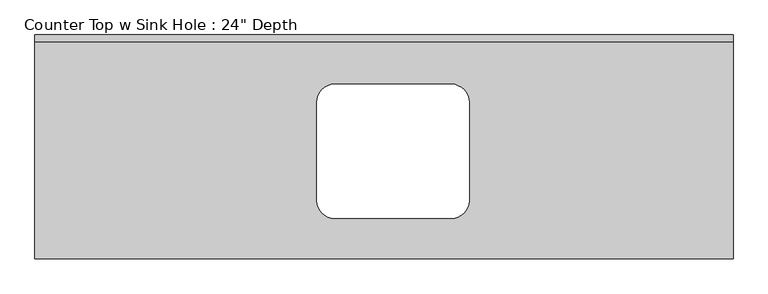
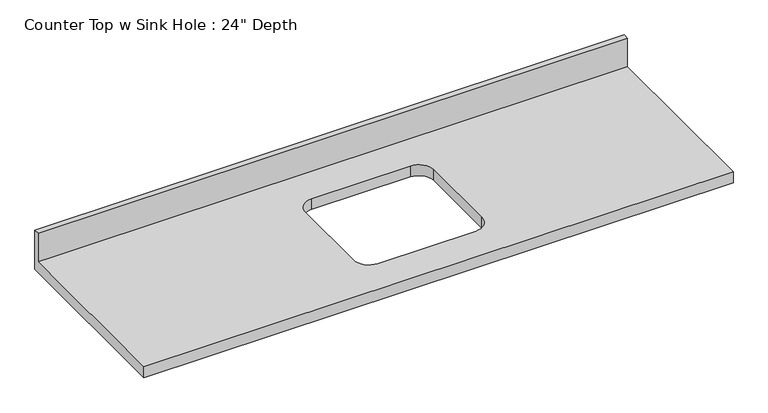
"""IFC4 building model written with IfcOpenShell, lengths in millimetres: furniture geometry."""

from ifc_helpers import new_model, si_unit, frame, origin, place, context, project, spatial, polyline, circle_curve, source, transform, mapped, element, save
from ifc_brep_helpers import plane_surface, revolved_surface, advanced_brep


def furniture_c6510c7c(model_context):
    return source(origin(), model_context, "Body", "AdvancedBrep", [
        advanced_brep(
        [(-1200.4622951, -635.0, 914.4), (780.7377049, -635.0, 914.4), (780.7377049, -19.05, 914.4), (-1200.4622951, -19.05, 914.4), (-349.5622951, -139.7, 914.4), (-19.3622951, -139.7, 914.4), (31.4377049, -190.5, 914.4), (31.4377049, -469.9, 914.4), (-19.3622951, -520.7, 914.4), (-349.5622951, -520.7, 914.4), (-400.3622951, -469.9, 914.4), (-400.3622951, -190.5, 914.4), (780.7377049, 0.0, 876.3), (780.7377049, -635.0, 876.3), (-1200.4622951, -635.0, 876.3), (-1200.4622951, 0.0, 876.3), (-19.3622951, -139.7, 876.3), (-349.5622951, -139.7, 876.3), (-400.3622951, -190.5, 876.3), (-400.3622951, -469.9, 876.3), (-349.5622951, -520.7, 876.3), (-19.3622951, -520.7, 876.3), (31.4377049, -469.9, 876.3), (31.4377049, -190.5, 876.3), (-1200.4622951, 0.0, 1016.0), (780.7377049, 0.0, 1016.0), (-1200.4622951, -19.05, 1016.0), (780.7377049, -19.05, 1016.0)],
        [
            (0, 1),
            (1, 2),
            (2, 3),
            (3, 0),
            (4, 5),
            (5, 6, circle_curve(frame((-19.3622951, -190.5, 914.4), z_axis=(0.0, 0.0, -1.0), x_axis=(1.0, 0.0, 0.0)), 50.8)),
            (6, 7),
            (7, 8, circle_curve(frame((-19.3622951, -469.9, 914.4), z_axis=(0.0, 0.0, -1.0), x_axis=(1.0, 0.0, 0.0)), 50.8)),
            (8, 9),
            (9, 10, circle_curve(frame((-349.5622951, -469.9, 914.4), z_axis=(0.0, 0.0, -1.0), x_axis=(1.0, 0.0, 0.0)), 50.8)),
            (10, 11),
            (11, 4, circle_curve(frame((-349.5622951, -190.5, 914.4), z_axis=(0.0, 0.0, -1.0), x_axis=(1.0, 0.0, 0.0)), 50.8)),
            (12, 13),
            (13, 14),
            (14, 15),
            (15, 12),
            (16, 17),
            (17, 18, circle_curve(frame((-349.5622951, -190.5, 876.3), z_axis=(0.0, 0.0, 1.0), x_axis=(1.0, 0.0, 0.0)), 50.8)),
            (18, 19),
            (19, 20, circle_curve(frame((-349.5622951, -469.9, 876.3), z_axis=(0.0, 0.0, 1.0), x_axis=(1.0, 0.0, 0.0)), 50.8)),
            (20, 21),
            (21, 22, circle_curve(frame((-19.3622951, -469.9, 876.3), z_axis=(0.0, 0.0, 1.0), x_axis=(1.0, 0.0, 0.0)), 50.8)),
            (22, 23),
            (23, 16, circle_curve(frame((-19.3622951, -190.5, 876.3), z_axis=(0.0, 0.0, 1.0), x_axis=(1.0, 0.0, 0.0)), 50.8)),
            (15, 24),
            (24, 25),
            (25, 12),
            (14, 0),
            (3, 26),
            (26, 24),
            (13, 1),
            (25, 27),
            (27, 2),
            (4, 17),
            (16, 5),
            (11, 18),
            (10, 19),
            (9, 20),
            (8, 21),
            (7, 22),
            (6, 23),
            (26, 27),
        ],
        [
            plane_surface(frame((-1200.4622951, 0.0, 914.4), z_axis=(0.0, 0.0, 1.0), x_axis=(-1.0, 0.0, 0.0))),
            plane_surface(frame((-1200.4622951, 0.0, 876.3), z_axis=(0.0, 0.0, -1.0), x_axis=(1.0, 0.0, 0.0))),
            plane_surface(frame((780.7377049, 0.0, 914.4), z_axis=(0.0, 1.0, 0.0), x_axis=(0.0, 0.0, -1.0))),
            plane_surface(frame((-1200.4622951, 0.0, 914.4), z_axis=(-1.0, 0.0, 0.0), x_axis=(0.0, 0.0, -1.0))),
            plane_surface(frame((-1200.4622951, -635.0, 914.4), z_axis=(0.0, -1.0, 0.0), x_axis=(0.0, 0.0, -1.0))),
            plane_surface(frame((780.7377049, -635.0, 914.4), z_axis=(1.0, 0.0, 0.0), x_axis=(0.0, 0.0, -1.0))),
            plane_surface(frame((-19.3622951, -139.7, 914.4), z_axis=(0.0, -1.0, 0.0), x_axis=(0.0, 0.0, -1.0))),
            revolved_surface(polyline([(-298.76229509999996, -190.5, 914.4), (-298.76229509999996, -190.5, 876.3)]), (-349.5622951, -190.5, 876.3), (0.0, 0.0, 1.0)),
            plane_surface(frame((-400.3622951, -190.5, 914.4), z_axis=(1.0, 0.0, 0.0), x_axis=(0.0, 0.0, -1.0))),
            revolved_surface(polyline([(-298.76229509999996, -469.9, 914.4), (-298.76229509999996, -469.9, 876.3)]), (-349.5622951, -469.9, 876.3), (0.0, 0.0, 1.0)),
            plane_surface(frame((-349.5622951, -520.7, 914.4), z_axis=(0.0, 1.0, 0.0), x_axis=(0.0, 0.0, -1.0))),
            revolved_surface(polyline([(31.437704899999996, -469.9, 914.4), (31.437704899999996, -469.9, 876.3)]), (-19.3622951, -469.9, 876.3), (0.0, 0.0, 1.0)),
            plane_surface(frame((31.4377049, -469.9, 914.4), z_axis=(-1.0, 0.0, 0.0), x_axis=(0.0, 0.0, -1.0))),
            revolved_surface(polyline([(31.437704899999996, -190.5, 914.4), (31.437704899999996, -190.5, 876.3)]), (-19.3622951, -190.5, 876.3), (0.0, 0.0, 1.0)),
            plane_surface(frame((-1200.4622951, 0.0, 1016.0), z_axis=(0.0, 0.0, 1.0), x_axis=(0.0, -1.0, 0.0))),
            plane_surface(frame((-1200.4622951, -19.05, 1016.0), z_axis=(0.0, -1.0, 0.0), x_axis=(0.0, 0.0, -1.0))),
        ],
        [
            (0, [[1, 2, 3, 4], [5, 6, 7, 8, 9, 10, 11, 12]]),
            (1, [[13, 14, 15, 16], [17, 18, 19, 20, 21, 22, 23, 24]]),
            (2, [[-16, 25, 26, 27]]),
            (3, [[-15, 28, -4, 29, 30, -25]]),
            (4, [[-1, -28, -14, 31]]),
            (5, [[-13, -27, 32, 33, -2, -31]]),
            (6, [[34, -17, 35, -5]]),
            (7, [[-34, -12, 36, -18]]),
            (8, [[-36, -11, 37, -19]]),
            (9, [[-37, -10, 38, -20]]),
            (10, [[-38, -9, 39, -21]]),
            (11, [[-39, -8, 40, -22]]),
            (12, [[-40, -7, 41, -23]]),
            (13, [[-35, -24, -41, -6]]),
            (14, [[-30, 42, -32, -26]]),
            (15, [[-42, -29, -3, -33]]),
        ],
    ),
    ])


if __name__ == "__main__":
    model = new_model("IFC4")
    model_context = context("Model", 3, world=origin())
    ifc_project = project(units=[si_unit("LENGTHUNIT", "METRE", prefix="MILLI")], contexts=[model_context])
    site = spatial("IfcSite", under=ifc_project)
    building = spatial("IfcBuilding", under=site)
    placement = place(None, origin())
    furniture_shape = furniture_c6510c7c(model_context)
    element("IfcFurniture", 1, ObjectType="Counter Top w Sink Hole : 24\" Depth", at=placement, inside=building, context=model_context, shape_type="MappedRepresentation", body=[
        mapped(furniture_shape, transform((0.0, 0.0, 0.0), x_axis=(1.0, 0.0, 0.0), y_axis=(0.0, 1.0, 0.0), z_axis=(0.0, 0.0, 1.0))),
    ])
    save(model, "model.ifc")

# Revit data of these elements
# Type "Counter Top w Sink Hole : 24\" Depth"
#   Assembly Code = "C1030400"
#   Counter Thickness = 0' - 1 1/2"
#   Depth = 2' - 1"
#   Height = 3' - 0"
#   Length [instance default] = 8' - 0"
#   Sink Location [instance default] = 2' - 0"
#   Sink Location To Wall [instance default] = 0' - 6"
#   Sink Opening Depth [instance default] = 1' - 3"
#   Sink Opening Width [instance default] = 2' - 3"
#   Counter Top Material = none
#   Default Elevation = 0
# Element 1 (IfcFurniture, "Counter Top w Sink Hole : 24\" Depth")
#   Length = 6' - 6"
#   Sink Location = 3' - 4"
#   Sink Opening Depth = 1' - 2"
#   Sink Opening Width = 1' - 4"
#   Materials on its faces: "Counter Top"
# Materials
#   "Counter Top": class "Wood", colour RGB 226 177 128, transparency 0
